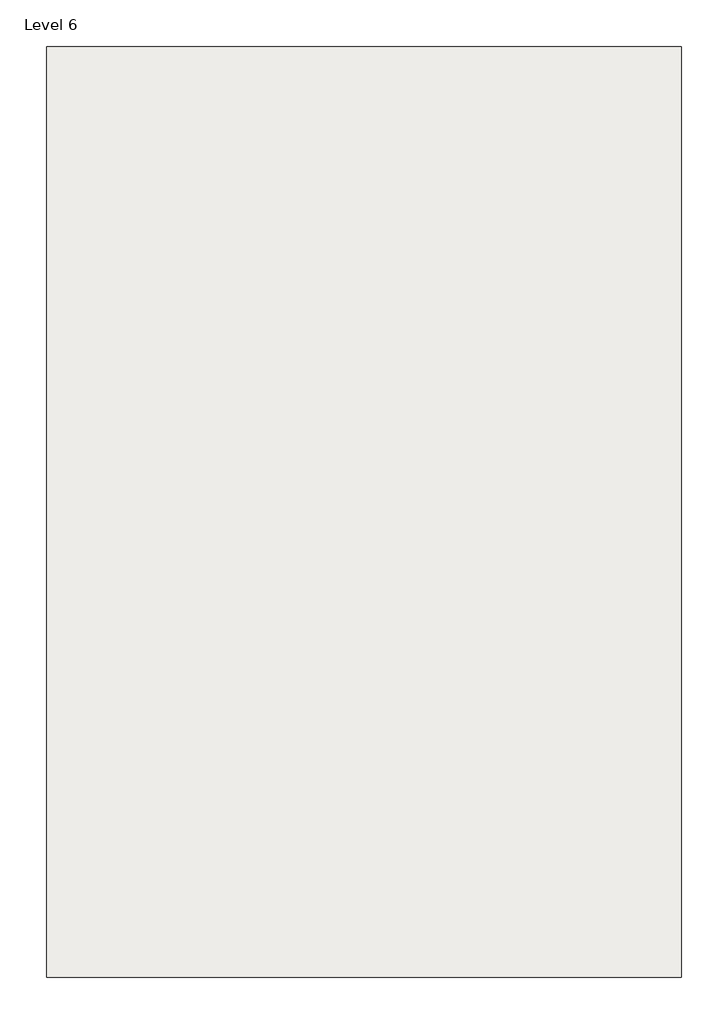
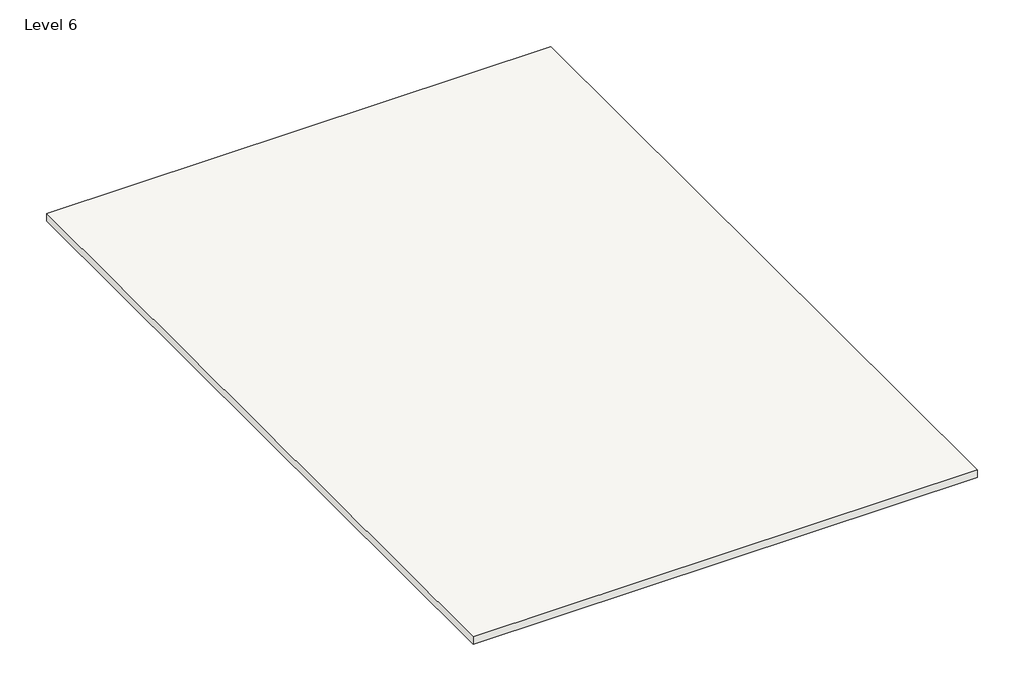
# One storey, incomplete: 1 roof.
"""IFC4 building model written with IfcOpenShell, lengths in millimetres."""

from ifc_helpers import new_model, si_unit, frame, origin, place, context, project, spatial, polyline, outline, extrude, element, save

model = new_model("IFC4")

# Units and contexts
model_context = context("Model", 3, world=origin())
ifc_project = project(units=[si_unit("LENGTHUNIT", "METRE", prefix="MILLI")], contexts=[model_context])

# Site, building, storey
site = spatial("IfcSite", under=ifc_project)
building = spatial("IfcBuilding", under=site)
storey = spatial("IfcBuildingStorey", under=building, Name="Level 6", Elevation=12801.6)

# Roof
placement = place(None, origin())
element("IfcRoof", 1, ObjectType="Generic - 12\"", at=placement, inside=storey, context=model_context, shape_type="SweptSolid", body=[
    extrude(outline(polyline([(-5991.4247832, 7671.8032079), (3647.8752168, 7671.8032079), (3647.8752168, -6450.5967921), (-5991.4247832, -6450.5967921), (-5991.4247832, 7671.8032079)])), frame((0.0, 0.0, 12649.2), z_axis=(0.0, 0.0, 1.0), x_axis=(1.0, 0.0, 0.0)), (0.0, 0.0, 1.0), 152.4),
])

save(model, "model.ifc")

# Revit data of these elements
# Type "Generic - 12\""
#   Assembly Code = "B1020"
#   Layers, outside or top first: 0' - 6" no material (function 1)
# Element 1 (IfcRoof, "Generic - 12\"")
#   built-in parameter 1001705 = 42 (stored number, unit not read)
#   built-in parameter 1001701 = -0.5 (stored number, unit not read)
#   built-in parameter 1001710 = 33615
#   Phase Created = New Construction
#   Materials on its faces: "Default Roof"
# Materials
#   "Default Roof": colour RGB 88 101 114, transparency 0, Cost = 0
